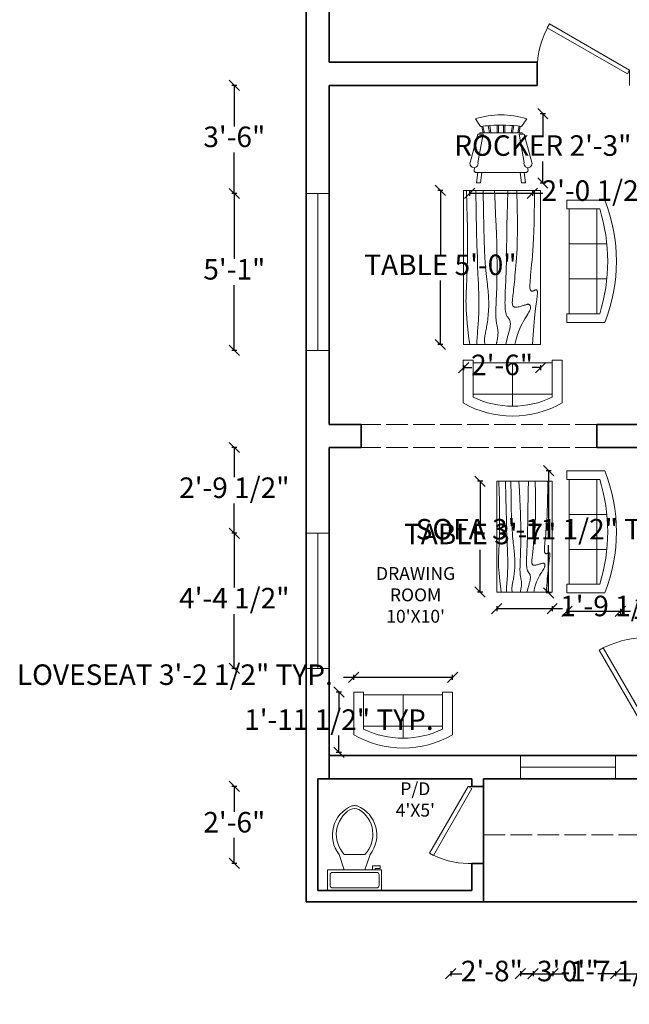
# Model space of a CAD drawing. Units: inches. Extents: x 2558 to 3026, y 433 to 1053.
# Tile 1 of 8: x 2558 to 2795, y 433 to 816. Entities that reach past the tile are written whole.
import ezdxf

# ---------------------------------------------------------------- set-up
doc = ezdxf.new("R2010")
doc.units = ezdxf.units.IN
doc.linetypes.add('ACAD_ISO02W100', pattern=[15, 12, -3])
for name, color, linetype, lineweight in [('A-ANNO-DIMS', 2, 'Continuous', 18), ('A-AREA-IDEN', 7, 'Continuous', 18), ('A-DOOR', 4, 'Continuous', 18), ('A-FLOR-FIXT', 9, 'Continuous', 18), ('A-FLOR-OVHD', 7, 'ACAD_ISO02W100', 18), ('A-FURN', 8, 'Continuous', 18), ('A-GLAZ', 5, 'Continuous', 18), ('A-WALL', 7, 'Continuous', 35), ('L-PLNT-BNDY', 253, 'ACAD_ISO02W100', 18)]:
    doc.layers.add(name, color=color, linetype=linetype, lineweight=lineweight)
doc.styles.get("Standard").update_dxf_attribs({"font": 'arial.ttf'})
doc.dimstyles.new('ISO-25', dxfattribs={"dimtxt": 8, "dimasz": 4, "dimexe": 1, "dimexo": 1, "dimgap": 1, "dimtad": 0, "dimtih": 1, "dimtoh": 1, "dimlunit": 3, "dimtxsty": 'Standard', "dimblk": 'OBLIQUE', "dimcen": 2.5, "dimclrt": 1, "dimadec": 0, "dimazin": 0, "dimtfac": 1, "dimtmove": 0, "dimatfit": 3, "dimfxl": 1, "dimfxlon": 1, "dimarcsym": 0})

# ---------------------------------------------------------------- blocks, each defined once
blk = doc.blocks.new('*U9')
for p, q in [((0, 0), (0, -6)), ((-36, 0), (-36, -6))]:
    blk.add_line(p, q)
blk.add_lwpolyline([(0, 0), (-31.18, 18), (-32.05, 16.48), (-0.88, -1.52)], close=True)
blk.add_arc((0, 0), 36, 150, 180)
blk = doc.blocks.new('*U8')
for p, q in [((0, 0), (0, -6)), ((36, 0), (36, -6))]:
    blk.add_line(p, q)
blk.add_lwpolyline([(0, 0), (31.18, 18), (32.05, 16.48), (0.87, -1.52)], close=True)
blk.add_arc((0, 0), 36, 0, 30)
blk = doc.blocks.new('*U5')
for p, q in [((0, 0), (0, 6)), ((30, 0), (30, 6))]:
    blk.add_line(p, q)
blk.add_lwpolyline([(0, 0), (25.98, -15), (26.86, -13.48), (0.87, 1.52)], close=True)
blk.add_arc((0, 0), 30, 330, 0)
blk = doc.blocks.new('Sofa - Roundback 7 ft.')
for p, q in [((-12.00002, -32.4421), (-12.00003, -6.5971)), ((11.99997, -32.4421), (11.99998, -6.5971)), ((-36.000027, -34), (-36.000027, -11.4696)), ((-35.999844, -13.3819), (35.9998, -13.3819)), ((35.99998, -34), (35.99998, -11.4696)), ((-36.000027, -32.4421), (35.99998, -32.4421))]:
    blk.add_line(p, q)
for points in [[(-36.000027, -34), (-42.000027, -34), (-42.000027, -8)], [(41.99998, -8), (41.99998, -34), (35.99998, -34)]]:
    blk.add_lwpolyline(points)
for centre, radius, start, end in [((0, -114.25), 114.25, 68.43141, 111.5686), ((-0.00001, -127.1968), 121.1968, 72.72033, 107.2797)]:
    blk.add_arc(centre, radius, start, end)
blk = doc.blocks.new('Sofa - Roundback Loveseat 5 ft.')
for p, q in [((-24, -33.99998), (-24, -11.46958)), ((0, -32.44198), (0, -5.99998)), ((24.00004, -33.99998), (24.00004, -11.46958)), ((-23.9998, -13.38178), (23.99986, -13.38178)), ((-24, -32.44198), (24.00004, -32.44198))]:
    blk.add_line(p, q)
for points in [[(-24, -33.99998), (-30, -33.99998), (-30, -7.99998)], [(30.00004, -7.99998), (30.00004, -33.99998), (24.00004, -33.99998)]]:
    blk.add_lwpolyline(points)
for centre, radius, start, end in [((0, -60.24998), 60.24998, 60.13715, 119.8628), ((0, -61.38438), 55.38444, 64.32083, 115.6792)]:
    blk.add_arc(centre, radius, start, end)
blk = doc.blocks.new('Chair - Rocking')
for p, q in [((-8, -4.5), (-10, -1.5)), ((8, -4.5), (10, -1.5)), ((-9, -7.5), (-12, -18.49999)), ((-7, -7.5), (-9, -7.5)), ((-9, -18.49999), (-7, -7.5)), ((-8.23428, -6.99939), (-8.3093, -7.47958)), ((-8.23041, -7), (8.23915, -7)), ((-7.5, -4.5), (-7, -7)), ((-6.5, -7), (-7.02225, -4.43)), ((-4.5, -7), (-4.96674, -4.19951)), ((-4, -7), (-4.40532, -4.16272)), ((-1.5, -4.05012), (-1.5, -7)), ((-1, -7), (-1, -4.05012)), ((1, -7), (1, -4.04655)), ((1.5, -4.05012), (1.5, -7)), ((4, -7), (4.40187, -4.18694)), ((4.5, -7), (4.96761, -4.19437)), ((6.5, -7), (7, -4.4057)), ((7.5, -4.5), (7, -7)), ((7, -7.5), (9, -7.5)), ((9, -18.49999), (7, -7.5)), ((8.31071, -7.48854), (8.23449, -7.00073)), ((9, -7.5), (12, -18.49999)), ((-10.36644, -20.64523), (-10.5, -21.49999)), ((-9, -22.49999), (-9.5, -26.49999)), ((0, -22.49999), (-9.5, -22.49999)), ((-8, -26.49999), (-7.5, -22.49999)), ((0, -22.49999), (9.5, -22.49999)), ((8, -26.49999), (7.5, -22.49999)), ((9, -22.49999), (9.5, -26.49999)), ((10.5, -21.49999), (10.3575, -20.58798)), ((-9.5, -26.49999), (-8, -26.49999)), ((9.5, -26.49999), (8, -26.49999))]:
    blk.add_line(p, q)
for centre, radius, start, end in [((0, -34.08333), 34.08333, 72.93847, 107.0615), ((0, -68.25004), 64.25, 93.92211, 97.15267), ((0, -68.25004), 64.25, 82.84733, 93.92211), ((-10.5, -18.99999), 1.58114, 161.5651, 18.43495), ((10.5, -18.99999), 1.58114, 161.5651, 18.43495), ((-9.5, -21.49999), 1, 180, 270), ((9.5, -21.49999), 1, 270, 0)]:
    blk.add_arc(centre, radius, start, end)
blk = doc.blocks.new('Table - Rectangular Woodgrain 60 x 30 in.')
for p, q in [((0, 0), (0, -30)), ((60, 0), (0, 0)), ((60, -30), (60, 0)), ((0, -30), (60, -30))]:
    blk.add_line(p, q)
for points in [[(0, -2.4), (4.8155, -2.418), (9.0302, -2.4688), (12.709, -2.5477), (15.9167, -2.65), (18.7181, -2.7711), (21.1781, -2.9063), (23.3616, -3.0508), (25.3333, -3.2), (27.1477, -3.3495), (28.8172, -3.4958), (30.3437, -3.636), (31.7291, -3.7667), (32.9756, -3.8849), (34.0849, -3.9875), (35.059, -4.0714), (35.9, -4.1334), (36.6114, -4.1711), (37.2041, -4.1854), (37.6906, -4.1779), (38.0833, -4.15), (38.3948, -4.1034), (38.6375, -4.0396), (38.8239, -3.9602), (38.9666, -3.8667), (39.0764, -3.7608), (39.1573, -3.6448), (39.2116, -3.521), (39.2416, -3.3917), (39.2498, -3.2593), (39.2385, -3.1261), (39.21, -2.9944), (39.1666, -2.8667), (39.111, -2.7447), (39.0468, -2.6281), (38.978, -2.5163), (38.9083, -2.4083), (38.8418, -2.3035), (38.7823, -2.201), (38.7337, -2.1001), (38.7, -2), (38.6844, -1.9003), (38.6875, -1.8021), (38.7094, -1.707), (38.75, -1.6167), (38.8094, -1.5326), (38.8875, -1.4563), (38.9844, -1.3893), (39.1, -1.3333), (39.2351, -1.2896), (39.3937, -1.2583), (39.5804, -1.2396), (39.8, -1.2333), (40.057, -1.2396), (40.3562, -1.2583), (40.7023, -1.2896), (41.1, -1.3333), (41.5547, -1.3895), (42.0755, -1.4573), (42.6721, -1.5361), (43.3542, -1.625), (44.1316, -1.7233), (45.014, -1.8302), (46.0114, -1.9449), (47.1333, -2.0667), (48.3862, -2.1947), (49.7625, -2.3281), (51.2513, -2.4663), (52.8416, -2.6083), (54.5226, -2.7535), (56.2833, -2.9011), (58.1127, -3.0501), (60, -3.2)], [(0, -9.2), (6.5759, -9.0858), (11.9385, -9.0365), (16.2527, -9.0418), (19.6833, -9.0917), (22.3952, -9.1759), (24.5531, -9.2844), (26.322, -9.4069), (27.8666, -9.5333), (29.3241, -9.6553), (30.7203, -9.7719), (32.0532, -9.8837), (33.3208, -9.9917), (34.5213, -10.0965), (35.6526, -10.199), (36.7128, -10.2999), (37.7, -10.4), (38.6129, -10.4996), (39.4531, -10.5969), (40.223, -10.6895), (40.925, -10.775), (41.5613, -10.8512), (42.1344, -10.9156), (42.6465, -10.966), (43.1, -11), (43.4976, -11.0158), (43.8437, -11.0136), (44.143, -10.9942), (44.4, -10.9583), (44.6195, -10.9069), (44.8062, -10.8406), (44.9648, -10.7603), (45.1, -10.6667), (45.2155, -10.5598), (45.3114, -10.4365), (45.3871, -10.2929), (45.4416, -10.125), (45.4743, -9.929), (45.4844, -9.7011), (45.4709, -9.4371), (45.4333, -9.1333), (45.3716, -8.7883), (45.2896, -8.4104), (45.1919, -8.0107), (45.0833, -7.6), (44.9685, -7.1893), (44.8521, -6.7896), (44.7388, -6.4117), (44.6333, -6.0667), (44.54, -5.7628), (44.4614, -5.4979), (44.4001, -5.2675), (44.3583, -5.0667), (44.3384, -4.8909), (44.3427, -4.7354), (44.3736, -4.5956), (44.4333, -4.4667), (44.5236, -4.3453), (44.6427, -4.2333), (44.7884, -4.1339), (44.9583, -4.05), (45.1501, -3.9849), (45.3614, -3.9417), (45.59, -3.9234), (45.8333, -3.9333), (46.0915, -3.9749), (46.3734, -4.0531), (46.6906, -4.1736), (47.0542, -4.3417), (47.4756, -4.5629), (47.9661, -4.8427), (48.5372, -5.1866), (49.2, -5.6), (49.9676, -6.0844), (50.8594, -6.625), (51.8965, -7.2031), (53.1, -7.8), (54.491, -8.3969), (56.0906, -8.975), (57.9199, -9.5156), (60, -10)], [(0, -12.8), (5.1847, -12.9322), (9.6213, -13.0323), (13.3963, -13.1059), (16.5958, -13.1583), (19.3063, -13.1952), (21.614, -13.2219), (23.6054, -13.2439), (25.3666, -13.2667), (26.9728, -13.2947), (28.4531, -13.3281), (29.8256, -13.3663), (31.1083, -13.4083), (32.3191, -13.4535), (33.476, -13.501), (34.597, -13.5501), (35.7, -13.6), (36.7984, -13.6497), (37.8875, -13.6979), (38.9578, -13.743), (40, -13.7833), (41.0047, -13.8174), (41.9625, -13.8438), (42.864, -13.8607), (43.7, -13.8667), (44.4631, -13.8604), (45.1552, -13.8417), (45.7801, -13.8104), (46.3416, -13.7667), (46.8439, -13.7104), (47.2906, -13.6417), (47.6858, -13.5604), (48.0333, -13.4667), (48.3375, -13.3608), (48.6042, -13.2448), (48.8396, -13.121), (49.05, -12.9917), (49.2417, -12.8593), (49.4208, -12.7261), (49.5937, -12.5944), (49.7667, -12.4667), (49.9452, -12.3451), (50.1323, -12.2313), (50.3303, -12.1268), (50.5416, -12.0333), (50.7686, -11.9524), (51.0135, -11.8854), (51.2788, -11.8341), (51.5666, -11.8), (51.8785, -11.7843), (52.2116, -11.7865), (52.562, -11.8059), (52.926, -11.8417), (53.2998, -11.8931), (53.6795, -11.9594), (54.0614, -12.0397), (54.4416, -12.1333), (54.8223, -12.2401), (55.2293, -12.3625), (55.6942, -12.5037), (56.2489, -12.6667), (56.9251, -12.8547), (57.7545, -13.0708), (58.7689, -13.3182), (60, -13.6)], [(0, -18), (5.124, -17.7273), (9.6609, -17.5057), (13.6705, -17.3303), (17.2125, -17.1958), (20.3467, -17.0973), (23.1328, -17.0297), (25.6307, -16.9878), (27.9, -16.9667), (29.9928, -16.9617), (31.9302, -16.9703), (33.7254, -16.9907), (35.3917, -17.0208), (36.9423, -17.0588), (38.3906, -17.1026), (39.7499, -17.1503), (41.0333, -17.2), (42.2519, -17.2496), (43.4073, -17.2969), (44.4986, -17.3395), (45.525, -17.375), (46.4858, -17.4012), (47.3802, -17.4156), (48.2074, -17.416), (48.9667, -17.4), (49.6583, -17.3662), (50.2872, -17.3167), (50.8595, -17.2547), (51.3812, -17.1833), (51.8584, -17.1057), (52.2971, -17.025), (52.7034, -16.9443), (53.0833, -16.8667), (53.443, -16.7951), (53.789, -16.7313), (54.128, -16.6768), (54.4666, -16.6334), (54.8115, -16.6024), (55.1693, -16.5854), (55.5465, -16.5841), (55.95, -16.6), (56.3828, -16.6337), (56.8346, -16.6823), (57.2915, -16.7418), (57.7396, -16.8084), (58.165, -16.878), (58.5539, -16.9469), (58.8924, -17.0111), (59.1666, -17.0667), (59.3679, -17.1107), (59.5078, -17.1438), (59.6032, -17.1675), (59.6708, -17.1833), (59.7275, -17.193), (59.7901, -17.1979), (59.8753, -17.1998), (60, -17.2)], [(0, -22.4), (8.0098, -22.2501), (14.4094, -22.1011), (19.4168, -21.9535), (23.25, -21.8083), (26.1269, -21.6663), (28.2656, -21.5281), (29.884, -21.3947), (31.2, -21.2667), (32.3967, -21.1448), (33.5172, -21.0292), (34.5697, -20.9198), (35.5625, -20.8167), (36.5037, -20.7198), (37.4015, -20.6292), (38.2642, -20.5448), (39.1, -20.4667), (39.9164, -20.3951), (40.7187, -20.3313), (41.5117, -20.2768), (42.3, -20.2333), (43.0883, -20.2024), (43.8812, -20.1854), (44.6836, -20.1841), (45.5, -20.2), (46.3328, -20.234), (47.1747, -20.2844), (48.0163, -20.3488), (48.8479, -20.425), (49.66, -20.5106), (50.4429, -20.6031), (51.1872, -20.7004), (51.8833, -20.8), (52.5246, -20.8999), (53.1166, -20.9995), (53.6681, -21.0983), (54.1875, -21.1958), (54.6834, -21.2919), (55.1646, -21.3859), (55.6394, -21.4777), (56.1167, -21.5667), (56.6028, -21.6515), (57.0961, -21.7266), (57.5929, -21.7852), (58.0896, -21.8208), (58.5823, -21.8268), (59.0674, -21.7964), (59.5412, -21.723), (60, -21.6)], [(0, -25.2), (8.6355, -25.0504), (15.7026, -24.9031), (21.4049, -24.7606), (25.9458, -24.625), (29.529, -24.4988), (32.3578, -24.3844), (34.6359, -24.284), (36.5667, -24.2), (38.3213, -24.1341), (39.9417, -24.0854), (41.437, -24.0523), (42.8167, -24.0333), (44.0901, -24.0268), (45.2667, -24.0313), (46.3557, -24.0451), (47.3667, -24.0667), (48.309, -24.0947), (49.1928, -24.1287), (50.0284, -24.168), (50.826, -24.2125), (51.5959, -24.2617), (52.3483, -24.3151), (53.0935, -24.3725), (53.8417, -24.4334), (54.6009, -24.497), (55.3699, -24.561), (56.1454, -24.6226), (56.9239, -24.6792), (57.7021, -24.7279), (58.4764, -24.7662), (59.2435, -24.7911), (60, -24.8)], [(0, -28.8), (5.6867, -28.6681), (10.45, -28.5698), (14.407, -28.5012), (17.675, -28.4584), (20.3711, -28.4374), (22.6125, -28.4344), (24.5164, -28.4455), (26.2, -28.4667), (27.762, -28.4947), (29.2276, -28.5281), (30.6033, -28.5663), (31.8958, -28.6084), (33.1118, -28.6535), (34.2578, -28.7011), (35.3405, -28.7501), (36.3666, -28.8), (37.3443, -28.8497), (38.288, -28.8974), (39.2137, -28.9412), (40.1375, -28.9792), (41.0753, -29.0093), (42.0432, -29.0297), (43.0572, -29.0384), (44.1333, -29.0333), (45.2936, -29.0114), (46.5843, -28.9641), (48.0579, -28.8816), (49.7666, -28.7542), (51.7629, -28.5721), (54.0989, -28.3255), (56.8272, -28.0048), (60, -27.6)]]:
    blk.add_lwpolyline(points)
blk = doc.blocks.new('Toilet - top')
for p, q in [((9.5, -6), (9.5, -2)), ((-10, -8.5), (-8, -8.5)), ((-10, -9.5), (-10, -8.5)), ((-7, -9.5), (-10, -9.5)), ((-8, -8.5), (-8, -8)), ((-7, -8), (-7, -9.5)), ((-4, -8), (-6, -14)), ((4, -8), (6, -14)), ((4, -14), (-4, -14))]:
    blk.add_line(p, q)
blk.add_lwpolyline([(10.5, -8), (10.5, 0), (-10.5, 0), (-10.5, -8)], close=True)
for points in [[(-9.5, -2), (-9.5, -6)], [(8.5, -1), (-8.5, -1)], [(-8.5, -7), (8.5, -7)]]:
    blk.add_lwpolyline(points)
for centre, radius, start, end in [((-8.62, -1.88), 0.884, 81.8699, 188.1301), ((8.62, -1.88), 0.884, 351.8699, 98.1301), ((-8.62, -6.12), 0.884, 171.8699, 278.1301), ((8.62, -6.12), 0.884, 261.8699, 8.1301), ((3.52, -21.58), 12.17, 141.4691, 247.9714), ((4.2, -21.82), 11.33, 136.3677, 238.9468), ((-3.52, -21.58), 12.17, 292.0284, 38.5307), ((-4.2, -21.82), 11.33, 301.053, 43.6321), ((0, -27.88), 4, 245.7318, 294.2682), ((0, -29), 4, 254.8605, 285.1395)]:
    blk.add_arc(centre, radius, start, end)
blk = doc.blocks.new('_Oblique')
at = {"color": 0, "linetype": 'ByBlock', "lineweight": -2}
blk.add_line((-0.5, -0.5), (0.5, 0.5), dxfattribs=at)
blk = doc.blocks.new('*D27')
at = {"layer": 'A-ANNO-DIMS', "color": 0, "lineweight": -2, "transparency": 16777216}
for p, q in [((2764.96, 640.74), (2762.96, 640.74)), ((2763.96, 640.74), (2763.96, 622.08)), ((2763.96, 593.15), (2763.96, 611.8)), ((2764.96, 593.15), (2762.96, 593.15))]:
    blk.add_line(p, q, dxfattribs=at)
at = {"layer": 'Defpoints', "color": 0, "transparency": 16777216}
for p in [(2771.1, 640.74), (2763.96, 593.15), (2771.1, 593.15)]:
    blk.add_point(p, dxfattribs=at)
at = {"layer": 'A-ANNO-DIMS', "color": 0, "lineweight": -2, "transparency": 16777216, "xscale": 4, "yscale": 4, "zscale": 4}
for p, rotation in [((2763.96, 640.74), 90), ((2763.96, 593.15), 270)]:
    blk.add_blockref('_Oblique', p, dxfattribs=dict(at, rotation=rotation))
at = {"layer": 'A-ANNO-DIMS', "color": 1, "transparency": 16777216, "insert": (2763.96, 616.94), "char_height": 8, "attachment_point": 5}
blk.add_mtext('SOFA 3\'-11 1/2" TYP.', dxfattribs=at)
blk = doc.blocks.new('*D28')
at = {"layer": 'A-ANNO-DIMS', "color": 0, "lineweight": -2, "transparency": 16777216}
for p, q in [((2771.1, 587.01), (2771.1, 585.01)), ((2791.87, 587.01), (2791.87, 585.01)), ((2771.1, 586.01), (2791.87, 586.01)), ((2791.87, 586.01), (2795.87, 586.01))]:
    blk.add_line(p, q, dxfattribs=at)
at = {"layer": 'Defpoints', "color": 0, "transparency": 16777216}
for p in [(2771.1, 593.15), (2791.87, 593.15), (2791.87, 586.01)]:
    blk.add_point(p, dxfattribs=at)
at = {"layer": 'A-ANNO-DIMS', "color": 0, "lineweight": -2, "transparency": 16777216, "xscale": 4, "yscale": 4, "zscale": 4, "rotation": 180}
blk.add_blockref('_Oblique', (2771.1, 586.01), dxfattribs=at)
at = {"layer": 'A-ANNO-DIMS', "color": 0, "lineweight": -2, "transparency": 16777216, "xscale": 4, "yscale": 4, "zscale": 4}
blk.add_blockref('_Oblique', (2791.87, 586.01), dxfattribs=at)
at = {"layer": 'A-ANNO-DIMS', "color": 1, "transparency": 16777216, "insert": (2820.88, 586.01), "char_height": 8, "attachment_point": 5}
blk.add_mtext('1\'-9" TYP.', dxfattribs=at)
blk = doc.blocks.new('*D29')
at = {"layer": 'A-ANNO-DIMS', "color": 0, "lineweight": -2, "transparency": 16777216}
for p, q in [((2688.13, 560.29), (2684.13, 560.29)), ((2688.13, 559.29), (2688.13, 561.29)), ((2726.58, 560.29), (2688.13, 560.29)), ((2726.58, 559.29), (2726.58, 561.29))]:
    blk.add_line(p, q, dxfattribs=at)
at = {"layer": 'Defpoints', "color": 0, "transparency": 16777216}
for p in [(2688.13, 560.29), (2688.13, 554.53), (2726.58, 554.53)]:
    blk.add_point(p, dxfattribs=at)
at = {"layer": 'A-ANNO-DIMS', "color": 0, "lineweight": -2, "transparency": 16777216, "xscale": 4, "yscale": 4, "zscale": 4, "rotation": 180}
blk.add_blockref('_Oblique', (2688.13, 560.29), dxfattribs=at)
at = {"layer": 'A-ANNO-DIMS', "color": 0, "lineweight": -2, "transparency": 16777216, "xscale": 4, "yscale": 4, "zscale": 4}
blk.add_blockref('_Oblique', (2726.58, 560.29), dxfattribs=at)
at = {"layer": 'A-ANNO-DIMS', "color": 1, "transparency": 16777216, "insert": (2618.55, 560.29), "char_height": 8, "attachment_point": 5}
blk.add_mtext('LOVESEAT 3\'-2 1/2" TYP.', dxfattribs=at)
blk = doc.blocks.new('*D30')
at = {"layer": 'A-ANNO-DIMS', "color": 0, "lineweight": -2, "transparency": 16777216}
for p, q in [((2683.37, 554.53), (2681.37, 554.53)), ((2682.37, 554.53), (2682.37, 547.92)), ((2682.37, 531.04), (2682.37, 537.65)), ((2683.37, 531.04), (2681.37, 531.04))]:
    blk.add_line(p, q, dxfattribs=at)
at = {"layer": 'Defpoints', "color": 0, "transparency": 16777216}
for p in [(2688.13, 554.53), (2682.37, 531.04), (2688.13, 531.04)]:
    blk.add_point(p, dxfattribs=at)
at = {"layer": 'A-ANNO-DIMS', "color": 0, "lineweight": -2, "transparency": 16777216, "xscale": 4, "yscale": 4, "zscale": 4}
for p, rotation in [((2682.37, 554.53), 90), ((2682.37, 531.04), 270)]:
    blk.add_blockref('_Oblique', p, dxfattribs=dict(at, rotation=rotation))
at = {"layer": 'A-ANNO-DIMS', "color": 1, "transparency": 16777216, "insert": (2682.37, 542.78), "char_height": 8, "attachment_point": 5}
blk.add_mtext('1\'-11 1/2" TYP.', dxfattribs=at)
blk = doc.blocks.new('*D31')
at = {"layer": 'A-ANNO-DIMS', "color": 0, "lineweight": -2, "transparency": 16777216}
for p, q in [((2722.86, 749.93), (2720.86, 749.93)), ((2721.86, 749.93), (2721.86, 725.02)), ((2721.86, 689.93), (2721.86, 714.85)), ((2722.86, 689.93), (2720.86, 689.93))]:
    blk.add_line(p, q, dxfattribs=at)
at = {"layer": 'Defpoints', "color": 0, "transparency": 16777216}
for p in [(2730.86, 749.93), (2721.86, 689.93), (2730.86, 689.93)]:
    blk.add_point(p, dxfattribs=at)
at = {"layer": 'A-ANNO-DIMS', "color": 0, "lineweight": -2, "transparency": 16777216, "xscale": 4, "yscale": 4, "zscale": 4}
for p, rotation in [((2721.86, 749.93), 90), ((2721.86, 689.93), 270)]:
    blk.add_blockref('_Oblique', p, dxfattribs=dict(at, rotation=rotation))
at = {"layer": 'A-ANNO-DIMS', "color": 1, "transparency": 16777216, "insert": (2721.86, 719.93), "char_height": 8, "attachment_point": 5}
blk.add_mtext('TABLE 5\'-0"', dxfattribs=at)
blk = doc.blocks.new('*D32')
at = {"layer": 'A-ANNO-DIMS', "color": 0, "lineweight": -2, "transparency": 16777216}
for p, q in [((2730.86, 681.93), (2730.86, 679.93)), ((2730.86, 680.93), (2734.15, 680.93)), ((2760.86, 680.93), (2757.56, 680.93)), ((2760.86, 681.93), (2760.86, 679.93))]:
    blk.add_line(p, q, dxfattribs=at)
at = {"layer": 'Defpoints', "color": 0, "transparency": 16777216}
for p in [(2730.86, 689.93), (2760.86, 689.93), (2760.86, 680.93)]:
    blk.add_point(p, dxfattribs=at)
at = {"layer": 'A-ANNO-DIMS', "color": 0, "lineweight": -2, "transparency": 16777216, "xscale": 4, "yscale": 4, "zscale": 4, "rotation": 180}
blk.add_blockref('_Oblique', (2730.86, 680.93), dxfattribs=at)
at = {"layer": 'A-ANNO-DIMS', "color": 0, "lineweight": -2, "transparency": 16777216, "xscale": 4, "yscale": 4, "zscale": 4}
blk.add_blockref('_Oblique', (2760.86, 680.93), dxfattribs=at)
at = {"layer": 'A-ANNO-DIMS', "color": 1, "transparency": 16777216, "insert": (2745.86, 680.93), "char_height": 8, "attachment_point": 5}
blk.add_mtext('2\'-6"', dxfattribs=at)
blk = doc.blocks.new('*D33')
at = {"layer": 'A-ANNO-DIMS', "color": 0, "lineweight": -2, "transparency": 16777216}
for p, q in [((2738.31, 636.64), (2736.31, 636.64)), ((2737.31, 636.64), (2737.31, 620.17)), ((2737.31, 593.52), (2737.31, 609.99)), ((2738.31, 593.52), (2736.31, 593.52))]:
    blk.add_line(p, q, dxfattribs=at)
at = {"layer": 'Defpoints', "color": 0, "transparency": 16777216}
for p in [(2743.78, 636.64), (2737.31, 593.52), (2743.78, 593.52)]:
    blk.add_point(p, dxfattribs=at)
at = {"layer": 'A-ANNO-DIMS', "color": 0, "lineweight": -2, "transparency": 16777216, "xscale": 4, "yscale": 4, "zscale": 4}
for p, rotation in [((2737.31, 636.64), 90), ((2737.31, 593.52), 270)]:
    blk.add_blockref('_Oblique', p, dxfattribs=dict(at, rotation=rotation))
at = {"layer": 'A-ANNO-DIMS', "color": 1, "transparency": 16777216, "insert": (2737.31, 615.08), "char_height": 8, "attachment_point": 5}
blk.add_mtext('TABLE 3\'-7"', dxfattribs=at)
blk = doc.blocks.new('*D34')
at = {"layer": 'A-ANNO-DIMS', "color": 0, "lineweight": -2, "transparency": 16777216}
for p, q in [((2743.78, 588.05), (2743.78, 586.05)), ((2743.78, 587.05), (2765.34, 587.05)), ((2765.34, 588.05), (2765.34, 586.05)), ((2765.34, 587.05), (2769.34, 587.05))]:
    blk.add_line(p, q, dxfattribs=at)
at = {"layer": 'Defpoints', "color": 0, "transparency": 16777216}
for p in [(2743.78, 593.52), (2765.34, 593.52), (2765.34, 587.05)]:
    blk.add_point(p, dxfattribs=at)
at = {"layer": 'A-ANNO-DIMS', "color": 0, "lineweight": -2, "transparency": 16777216, "xscale": 4, "yscale": 4, "zscale": 4, "rotation": 180}
blk.add_blockref('_Oblique', (2743.78, 587.05), dxfattribs=at)
at = {"layer": 'A-ANNO-DIMS', "color": 0, "lineweight": -2, "transparency": 16777216, "xscale": 4, "yscale": 4, "zscale": 4}
blk.add_blockref('_Oblique', (2765.34, 587.05), dxfattribs=at)
at = {"layer": 'A-ANNO-DIMS', "color": 1, "transparency": 16777216, "insert": (2789.92, 587.05), "char_height": 8, "attachment_point": 5}
blk.add_mtext('1\'-9 1/2"', dxfattribs=at)
blk = doc.blocks.new('*D39')
at = {"layer": 'A-ANNO-DIMS', "color": 0, "lineweight": -2, "transparency": 16777216}
for p, q in [((2760.72, 779.87), (2762.72, 779.87)), ((2761.72, 779.87), (2761.72, 771.51)), ((2761.72, 752.87), (2761.72, 761.23)), ((2760.72, 752.87), (2762.72, 752.87))]:
    blk.add_line(p, q, dxfattribs=at)
at = {"layer": 'Defpoints', "color": 0, "transparency": 16777216}
for p in [(2757.67, 779.87), (2761.72, 779.87), (2757.67, 752.87)]:
    blk.add_point(p, dxfattribs=at)
at = {"layer": 'A-ANNO-DIMS', "color": 0, "lineweight": -2, "transparency": 16777216, "xscale": 4, "yscale": 4, "zscale": 4}
for p, rotation in [((2761.72, 779.87), 90), ((2761.72, 752.87), 270)]:
    blk.add_blockref('_Oblique', p, dxfattribs=dict(at, rotation=rotation))
at = {"layer": 'A-ANNO-DIMS', "color": 1, "transparency": 16777216, "insert": (2761.72, 766.37), "char_height": 8, "attachment_point": 5}
blk.add_mtext('ROCKER 2\'-3"', dxfattribs=at)
blk = doc.blocks.new('*D40')
at = {"layer": 'A-ANNO-DIMS', "color": 0, "lineweight": -2, "transparency": 16777216}
for p, q in [((2733.24, 749.82), (2733.24, 747.82)), ((2733.24, 748.82), (2757.67, 748.82)), ((2757.67, 749.82), (2757.67, 747.82)), ((2757.67, 748.82), (2761.67, 748.82))]:
    blk.add_line(p, q, dxfattribs=at)
at = {"layer": 'Defpoints', "color": 0, "transparency": 16777216}
for p in [(2733.24, 752.87), (2757.67, 752.87), (2757.67, 748.82)]:
    blk.add_point(p, dxfattribs=at)
at = {"layer": 'A-ANNO-DIMS', "color": 0, "lineweight": -2, "transparency": 16777216, "xscale": 4, "yscale": 4, "zscale": 4, "rotation": 180}
blk.add_blockref('_Oblique', (2733.24, 748.82), dxfattribs=at)
at = {"layer": 'A-ANNO-DIMS', "color": 0, "lineweight": -2, "transparency": 16777216, "xscale": 4, "yscale": 4, "zscale": 4}
blk.add_blockref('_Oblique', (2757.67, 748.82), dxfattribs=at)
at = {"layer": 'A-ANNO-DIMS', "color": 1, "transparency": 16777216, "insert": (2782.69, 748.82), "char_height": 8, "attachment_point": 5}
blk.add_mtext('2\'-0 1/2"', dxfattribs=at)
blk = doc.blocks.new('*D48')
at = {"layer": 'A-ANNO-DIMS', "color": 0, "lineweight": -2, "transparency": 16777216}
for p, q in [((2725.89, 445.87), (2725.89, 443.87)), ((2725.89, 444.87), (2730.19, 444.87)), ((2757.89, 444.87), (2753.59, 444.87)), ((2757.89, 445.87), (2757.89, 443.87))]:
    blk.add_line(p, q, dxfattribs=at)
at = {"layer": 'Defpoints', "color": 0, "transparency": 16777216}
for p in [(2725.89, 943.82), (2757.89, 943.82), (2757.89, 444.87)]:
    blk.add_point(p, dxfattribs=at)
at = {"layer": 'A-ANNO-DIMS', "color": 0, "lineweight": -2, "transparency": 16777216, "xscale": 4, "yscale": 4, "zscale": 4, "rotation": 180}
blk.add_blockref('_Oblique', (2725.89, 444.87), dxfattribs=at)
at = {"layer": 'A-ANNO-DIMS', "color": 0, "lineweight": -2, "transparency": 16777216, "xscale": 4, "yscale": 4, "zscale": 4}
blk.add_blockref('_Oblique', (2757.89, 444.87), dxfattribs=at)
at = {"layer": 'A-ANNO-DIMS', "color": 1, "transparency": 16777216, "insert": (2741.89, 444.87), "char_height": 8, "attachment_point": 5}
blk.add_mtext('2\'-8"', dxfattribs=at)
blk = doc.blocks.new('*D51')
at = {"layer": 'A-ANNO-DIMS', "color": 0, "lineweight": -2, "transparency": 16777216}
for p, q in [((2642.68, 517.82), (2640.68, 517.82)), ((2641.68, 517.82), (2641.68, 507.91)), ((2641.68, 487.82), (2641.68, 497.74)), ((2642.68, 487.82), (2640.68, 487.82))]:
    blk.add_line(p, q, dxfattribs=at)
at = {"layer": 'Defpoints', "color": 0, "transparency": 16777216}
for p in [(2641.68, 517.82), (2734.13, 517.82), (2734.13, 487.82)]:
    blk.add_point(p, dxfattribs=at)
at = {"layer": 'A-ANNO-DIMS', "color": 0, "lineweight": -2, "transparency": 16777216, "xscale": 4, "yscale": 4, "zscale": 4}
for p, rotation in [((2641.68, 517.82), 90), ((2641.68, 487.82), 270)]:
    blk.add_blockref('_Oblique', p, dxfattribs=dict(at, rotation=rotation))
at = {"layer": 'A-ANNO-DIMS', "color": 1, "transparency": 16777216, "insert": (2641.68, 502.82), "char_height": 8, "attachment_point": 5}
blk.add_mtext('2\'-6"', dxfattribs=at)
blk = doc.blocks.new('*D54')
at = {"layer": 'A-ANNO-DIMS', "color": 0, "lineweight": -2, "transparency": 16777216}
for p, q in [((2642.68, 748.74), (2640.68, 748.74)), ((2641.68, 748.74), (2641.68, 723.26)), ((2641.68, 687.61), (2641.68, 713.09)), ((2642.68, 687.61), (2640.68, 687.61))]:
    blk.add_line(p, q, dxfattribs=at)
at = {"layer": 'Defpoints', "color": 0, "transparency": 16777216}
for p in [(2641.68, 748.74), (2669.63, 748.74), (2669.63, 687.61)]:
    blk.add_point(p, dxfattribs=at)
at = {"layer": 'A-ANNO-DIMS', "color": 0, "lineweight": -2, "transparency": 16777216, "xscale": 4, "yscale": 4, "zscale": 4}
for p, rotation in [((2641.68, 748.74), 90), ((2641.68, 687.61), 270)]:
    blk.add_blockref('_Oblique', p, dxfattribs=dict(at, rotation=rotation))
at = {"layer": 'A-ANNO-DIMS', "color": 1, "transparency": 16777216, "insert": (2641.68, 718.17), "char_height": 8, "attachment_point": 5}
blk.add_mtext('5\'-1"', dxfattribs=at)
blk = doc.blocks.new('*D56')
at = {"layer": 'A-ANNO-DIMS', "color": 0, "lineweight": -2, "transparency": 16777216}
for p, q in [((2642.68, 616.4), (2640.68, 616.4)), ((2641.68, 616.4), (2641.68, 595.23)), ((2641.68, 563.78), (2641.68, 584.95)), ((2642.68, 563.78), (2640.68, 563.78))]:
    blk.add_line(p, q, dxfattribs=at)
at = {"layer": 'Defpoints', "color": 0, "transparency": 16777216}
for p in [(2641.68, 616.4), (2669.63, 616.4), (2669.63, 563.78)]:
    blk.add_point(p, dxfattribs=at)
at = {"layer": 'A-ANNO-DIMS', "color": 0, "lineweight": -2, "transparency": 16777216, "xscale": 4, "yscale": 4, "zscale": 4}
for p, rotation in [((2641.68, 616.4), 90), ((2641.68, 563.78), 270)]:
    blk.add_blockref('_Oblique', p, dxfattribs=dict(at, rotation=rotation))
at = {"layer": 'A-ANNO-DIMS', "color": 1, "transparency": 16777216, "insert": (2641.68, 590.09), "char_height": 8, "attachment_point": 5}
blk.add_mtext('4\'-4 1/2"', dxfattribs=at)
blk = doc.blocks.new('*D57')
at = {"layer": 'A-ANNO-DIMS', "color": 0, "lineweight": -2, "transparency": 16777216}
for p, q in [((2752.98, 445.87), (2752.98, 443.87)), ((2752.98, 444.87), (2759.88, 444.87)), ((2790.04, 444.87), (2783.14, 444.87)), ((2790.04, 445.87), (2790.04, 443.87))]:
    blk.add_line(p, q, dxfattribs=at)
at = {"layer": 'Defpoints', "color": 0, "transparency": 16777216}
for p in [(2752.98, 520.82), (2790.04, 520.82), (2790.04, 444.87)]:
    blk.add_point(p, dxfattribs=at)
at = {"layer": 'A-ANNO-DIMS', "color": 0, "lineweight": -2, "transparency": 16777216, "xscale": 4, "yscale": 4, "zscale": 4, "rotation": 180}
blk.add_blockref('_Oblique', (2752.98, 444.87), dxfattribs=at)
at = {"layer": 'A-ANNO-DIMS', "color": 0, "lineweight": -2, "transparency": 16777216, "xscale": 4, "yscale": 4, "zscale": 4}
blk.add_blockref('_Oblique', (2790.04, 444.87), dxfattribs=at)
at = {"layer": 'A-ANNO-DIMS', "color": 1, "transparency": 16777216, "insert": (2771.51, 444.87), "char_height": 8, "attachment_point": 5}
blk.add_mtext('3\'-1"', dxfattribs=at)
blk = doc.blocks.new('*D59')
at = {"layer": 'A-ANNO-DIMS', "color": 0, "lineweight": -2, "transparency": 16777216}
for p, q in [((2690.99, 1039.77), (2690.99, 1041.77)), ((2690.99, 1040.77), (2715.93, 1040.77)), ((2782.72, 1040.77), (2757.77, 1040.77)), ((2782.72, 1039.77), (2782.72, 1041.77))]:
    blk.add_line(p, q, dxfattribs=at)
at = {"layer": 'Defpoints', "color": 0, "transparency": 16777216}
for p in [(2782.72, 1040.77), (2690.99, 658.82), (2782.72, 658.82)]:
    blk.add_point(p, dxfattribs=at)
at = {"layer": 'A-ANNO-DIMS', "color": 0, "lineweight": -2, "transparency": 16777216, "xscale": 4, "yscale": 4, "zscale": 4, "rotation": 180}
blk.add_blockref('_Oblique', (2690.99, 1040.77), dxfattribs=at)
at = {"layer": 'A-ANNO-DIMS', "color": 0, "lineweight": -2, "transparency": 16777216, "xscale": 4, "yscale": 4, "zscale": 4}
blk.add_blockref('_Oblique', (2782.72, 1040.77), dxfattribs=at)
at = {"layer": 'A-ANNO-DIMS', "color": 1, "transparency": 16777216, "insert": (2736.85, 1040.77), "char_height": 8, "attachment_point": 5}
blk.add_mtext('7\'-7 1/2"', dxfattribs=at)
blk = doc.blocks.new('*D63')
at = {"layer": 'A-ANNO-DIMS', "color": 0, "lineweight": -2, "transparency": 16777216}
for p, q in [((2757.89, 445.87), (2757.89, 443.87)), ((2757.89, 444.87), (2765.63, 444.87)), ((2765.63, 445.87), (2765.63, 443.87)), ((2765.63, 444.87), (2769.63, 444.87))]:
    blk.add_line(p, q, dxfattribs=at)
at = {"layer": 'Defpoints', "color": 0, "transparency": 16777216}
for p in [(2757.89, 943.82), (2765.63, 943.82), (2765.63, 444.87)]:
    blk.add_point(p, dxfattribs=at)
at = {"layer": 'A-ANNO-DIMS', "color": 0, "lineweight": -2, "transparency": 16777216, "xscale": 4, "yscale": 4, "zscale": 4, "rotation": 180}
blk.add_blockref('_Oblique', (2757.89, 444.87), dxfattribs=at)
at = {"layer": 'A-ANNO-DIMS', "color": 0, "lineweight": -2, "transparency": 16777216, "xscale": 4, "yscale": 4, "zscale": 4}
blk.add_blockref('_Oblique', (2765.63, 444.87), dxfattribs=at)
at = {"layer": 'A-ANNO-DIMS', "color": 1, "transparency": 16777216, "insert": (2790.59, 444.87), "char_height": 8, "attachment_point": 5}
blk.add_mtext('0\'-7 1/2"', dxfattribs=at)
blk = doc.blocks.new('*D66')
at = {"layer": 'A-ANNO-DIMS', "color": 0, "lineweight": -2, "transparency": 16777216}
for p, q in [((2642.68, 790.82), (2640.68, 790.82)), ((2641.68, 790.82), (2641.68, 774.87)), ((2641.68, 748.74), (2641.68, 764.69)), ((2642.68, 748.74), (2640.68, 748.74))]:
    blk.add_line(p, q, dxfattribs=at)
at = {"layer": 'Defpoints', "color": 0, "transparency": 16777216}
for p in [(2641.68, 790.82), (2678.63, 790.82), (2669.63, 748.74)]:
    blk.add_point(p, dxfattribs=at)
at = {"layer": 'A-ANNO-DIMS', "color": 0, "lineweight": -2, "transparency": 16777216, "xscale": 4, "yscale": 4, "zscale": 4}
for p, rotation in [((2641.68, 790.82), 90), ((2641.68, 748.74), 270)]:
    blk.add_blockref('_Oblique', p, dxfattribs=dict(at, rotation=rotation))
at = {"layer": 'A-ANNO-DIMS', "color": 1, "transparency": 16777216, "insert": (2641.68, 769.78), "char_height": 8, "attachment_point": 5}
blk.add_mtext('3\'-6"', dxfattribs=at)
blk = doc.blocks.new('*D68')
at = {"layer": 'A-ANNO-DIMS', "color": 0, "lineweight": -2, "transparency": 16777216}
for p, q in [((2642.68, 649.82), (2640.68, 649.82)), ((2641.68, 649.82), (2641.68, 638.25)), ((2641.68, 616.4), (2641.68, 627.98)), ((2642.68, 616.4), (2640.68, 616.4))]:
    blk.add_line(p, q, dxfattribs=at)
at = {"layer": 'Defpoints', "color": 0, "transparency": 16777216}
for p in [(2641.68, 649.82), (2678.63, 649.82), (2669.63, 616.4)]:
    blk.add_point(p, dxfattribs=at)
at = {"layer": 'A-ANNO-DIMS', "color": 0, "lineweight": -2, "transparency": 16777216, "xscale": 4, "yscale": 4, "zscale": 4}
for p, rotation in [((2641.68, 649.82), 90), ((2641.68, 616.4), 270)]:
    blk.add_blockref('_Oblique', p, dxfattribs=dict(at, rotation=rotation))
at = {"layer": 'A-ANNO-DIMS', "color": 1, "transparency": 16777216, "insert": (2641.68, 633.11), "char_height": 8, "attachment_point": 5}
blk.add_mtext('2\'-9 1/2"', dxfattribs=at)
blk = doc.blocks.new('*D69')
at = {"layer": 'A-ANNO-DIMS', "color": 0, "lineweight": -2, "transparency": 16777216}
for p, q in [((2790.04, 445.87), (2790.04, 443.87)), ((2790.04, 444.87), (2807.63, 444.87)), ((2807.63, 445.87), (2807.63, 443.87)), ((2807.63, 444.87), (2811.63, 444.87))]:
    blk.add_line(p, q, dxfattribs=at)
at = {"layer": 'Defpoints', "color": 0, "transparency": 16777216}
for p in [(2790.04, 520.82), (2807.63, 520.82), (2807.63, 444.87)]:
    blk.add_point(p, dxfattribs=at)
at = {"layer": 'A-ANNO-DIMS', "color": 0, "lineweight": -2, "transparency": 16777216, "xscale": 4, "yscale": 4, "zscale": 4, "rotation": 180}
blk.add_blockref('_Oblique', (2790.04, 444.87), dxfattribs=at)
at = {"layer": 'A-ANNO-DIMS', "color": 0, "lineweight": -2, "transparency": 16777216, "xscale": 4, "yscale": 4, "zscale": 4}
blk.add_blockref('_Oblique', (2807.63, 444.87), dxfattribs=at)
at = {"layer": 'A-ANNO-DIMS', "color": 1, "transparency": 16777216, "insert": (2832.21, 444.87), "char_height": 8, "attachment_point": 5}
blk.add_mtext('1\'-5 1/2"', dxfattribs=at)
blk = doc.blocks.new('*D70')
at = {"layer": 'A-ANNO-DIMS', "color": 0, "lineweight": -2, "transparency": 16777216}
for p, q in [((2678.63, 1039.77), (2678.63, 1041.77)), ((2678.63, 1040.77), (2690.99, 1040.77)), ((2690.99, 1039.77), (2690.99, 1041.77)), ((2690.99, 1040.77), (2694.99, 1040.77))]:
    blk.add_line(p, q, dxfattribs=at)
at = {"layer": 'Defpoints', "color": 0, "transparency": 16777216}
for p in [(2690.99, 1040.77), (2678.63, 658.82), (2690.99, 658.82)]:
    blk.add_point(p, dxfattribs=at)
at = {"layer": 'A-ANNO-DIMS', "color": 0, "lineweight": -2, "transparency": 16777216, "xscale": 4, "yscale": 4, "zscale": 4, "rotation": 180}
blk.add_blockref('_Oblique', (2678.63, 1040.77), dxfattribs=at)
at = {"layer": 'A-ANNO-DIMS', "color": 0, "lineweight": -2, "transparency": 16777216, "xscale": 4, "yscale": 4, "zscale": 4}
blk.add_blockref('_Oblique', (2690.99, 1040.77), dxfattribs=at)
at = {"layer": 'A-ANNO-DIMS', "color": 1, "transparency": 16777216, "insert": (2715.56, 1040.77), "char_height": 8, "attachment_point": 5}
blk.add_mtext('1\'-0 1/2"', dxfattribs=at)

msp = doc.modelspace()

# ---------------------------------------------------------------- linework, layer by layer
at = {"layer": 'A-FLOR-OVHD', "ltscale": 0.7}
for p, q in [((2782.721, 658.825), (2690.987, 658.825)), ((2782.721, 649.825), (2690.987, 649.825))]:
    msp.add_line(p, q, dxfattribs=at)
at = {"layer": 'A-GLAZ'}
for p, q in [((2678.633, 748.738), (2669.633, 748.738)), ((2674.133, 748.738), (2674.133, 687.608)), ((2678.633, 687.608), (2669.633, 687.608)), ((2678.633, 616.403), (2669.633, 616.403)), ((2674.133, 616.403), (2674.133, 563.778)), ((2678.633, 563.778), (2669.633, 563.778)), ((2752.982, 520.825), (2752.982, 529.825)), ((2790.035, 529.825), (2790.035, 520.825)), ((2752.982, 525.325), (2790.035, 525.325))]:
    msp.add_line(p, q, dxfattribs=at)
at = {"layer": 'A-WALL'}
for p, q in [((2669.633, 1012.825), (2669.633, 472.825)), ((2678.633, 943.825), (2678.633, 799.825)), ((2759.497, 799.825), (2678.633, 799.825)), ((2759.497, 790.825), (2759.497, 799.825)), ((2678.633, 790.825), (2678.633, 658.825)), ((2759.497, 790.825), (2678.633, 790.825)), ((2690.987, 658.825), (2678.633, 658.825)), ((2690.987, 658.825), (2690.987, 649.825)), ((2807.633, 658.825), (2782.721, 658.825)), ((2782.721, 649.825), (2782.721, 658.825)), ((2678.633, 649.825), (2678.633, 520.825)), ((2690.987, 649.825), (2678.633, 649.825)), ((2798.633, 649.825), (2782.721, 649.825)), ((2798.633, 529.825), (2678.633, 529.825)), ((2674.133, 520.825), (2674.133, 477.325)), ((2734.133, 520.825), (2674.133, 520.825)), ((2734.133, 520.825), (2734.133, 517.825)), ((2734.133, 517.825), (2738.633, 517.825)), ((2807.633, 520.825), (2738.633, 520.825)), ((2738.633, 520.825), (2738.633, 472.825)), ((2734.133, 487.825), (2738.633, 487.825)), ((2734.133, 487.825), (2734.133, 477.325)), ((2674.133, 477.325), (2734.133, 477.325)), ((2669.633, 472.825), (2969.633, 472.825))]:
    msp.add_line(p, q, dxfattribs=at)
at = {"layer": 'L-PLNT-BNDY', "ltscale": 0.7}
msp.add_line((2738.633, 498.947), (2960.633, 498.947), dxfattribs=at)

# ---------------------------------------------------------------- block references
at = {"layer": 'A-DOOR'}
msp.add_blockref('*U9', (2795.497, 796.825), dxfattribs=at)
for name, p, rotation in [('*U8', (2801.633, 539.691), 90), ('*U5', (2732.633, 517.825), 270)]:
    msp.add_blockref(name, p, dxfattribs=dict(at, rotation=rotation))
at = {"layer": 'A-FLOR-FIXT', "rotation": 180}
msp.add_blockref('Toilet - top', (2688.477, 477.325), dxfattribs=at)
at = {"layer": 'A-FURN'}
msp.add_blockref('Chair - Rocking', (2745.453, 779.371), dxfattribs=at)
at = {"layer": 'A-FURN', "rotation": 270}
msp.add_blockref('Table - Rectangular Woodgrain 60 x 30 in.', (2760.856, 749.933), dxfattribs=at)
at = {"layer": 'A-FURN'}
for name, p, xscale, yscale, zscale, rotation in [('Sofa - Roundback 7 ft.', (2790.362, 722.322), 0.5665475993370205, 0.5665475993370205, 0.5665475993370205, 270), ('Sofa - Roundback Loveseat 5 ft.', (2749.959, 662.045), 0.6406989062008118, 0.6406989062008118, 0.6406989062008118, 180), ('Sofa - Roundback 7 ft.', (2790.362, 616.943), 0.5665475993370205, 0.5665475993370205, 0.5665475993370205, 270), ('Table - Rectangular Woodgrain 60 x 30 in.', (2765.339, 636.641), 0.7186959398027013, 0.7186959398027013, 0.7186959398027013, 270), ('Sofa - Roundback Loveseat 5 ft.', (2707.355, 532.745), 0.6406989062008118, 0.6406989062008118, 0.6406989062008118, 180)]:
    msp.add_blockref(name, p, dxfattribs=dict(at, xscale=xscale, yscale=yscale, zscale=zscale, rotation=rotation))

# ---------------------------------------------------------------- texts
at = {"layer": 'A-AREA-IDEN', "char_height": 5, "attachment_point": 1}
for s, width, insert in [("\\pxqc;DRAWING ROOM\\P10'X10'", 50.35476, (2687.035, 603.24)), ("\\pxqc;P/D\\P4'X5'", 46.06135, (2689.073, 519.401))]:
    msp.add_mtext_dynamic_manual_height_columns(s, width=width, gutter_width=12.5, heights=[0], dxfattribs=dict(at, insert=insert))

# ---------------------------------------------------------------- dimensions: what is measured, and where the dimension line sits
at = {"layer": 'A-ANNO-DIMS'}
for base, p1, p2, picture, middle in [((2690.987, 1040.775), (2678.633, 658.825), (2690.987, 658.825), '*D70', (2715.564, 1040.775)), ((2782.721, 1040.775), (2690.987, 658.825), (2782.721, 658.825), '*D59', (2736.854, 1040.775)), ((2757.892, 444.875), (2725.892, 943.825), (2757.892, 943.825), '*D48', (2741.892, 444.875)), ((2765.633, 444.875), (2757.892, 943.825), (2765.633, 943.825), '*D63', (2790.586, 444.875)), ((2757.67, 748.821), (2733.235, 752.871), (2757.67, 752.871), '*D40', (2782.692, 748.821)), ((2760.856, 680.933), (2730.856, 689.933), (2760.856, 689.933), '*D32', (2745.856, 680.933)), ((2765.339, 587.051), (2743.778, 593.52), (2765.339, 593.52), '*D34', (2789.916, 587.051)), ((2790.035, 444.875), (2752.982, 520.825), (2790.035, 520.825), '*D57', (2771.509, 444.875)), ((2807.633, 444.875), (2790.035, 520.825), (2807.633, 520.825), '*D69', (2832.21, 444.875))]:
    dim = msp.add_linear_dim(base=base, p1=p1, p2=p2, dimstyle='ISO-25', override={"dimdec": 1, "dimlfac": 1, "dimrnd": 0, "dimzin": 1, "dimdsep": 46, "dimlunit": 4, "dimfrac": 2}, dxfattribs=at)
    dim.commit()
    dim.dimension.update_dxf_attribs({"geometry": picture, "text_midpoint": middle})
for base, p1, p2, picture, middle in [((2641.683, 790.825), (2669.633, 748.738), (2678.633, 790.825), '*D66', (2641.683, 769.781)), ((2641.683, 748.738), (2669.633, 687.608), (2669.633, 748.738), '*D54', (2641.683, 718.173)), ((2641.683, 649.825), (2669.633, 616.403), (2678.633, 649.825), '*D68', (2641.683, 633.114)), ((2641.683, 616.403), (2669.633, 563.778), (2669.633, 616.403), '*D56', (2641.683, 590.09)), ((2641.683, 517.825), (2734.133, 487.825), (2734.133, 517.825), '*D51', (2641.683, 502.825))]:
    dim = msp.add_linear_dim(base=base, p1=p1, p2=p2, angle=90, dimstyle='ISO-25', override={"dimdec": 1, "dimlfac": 1, "dimrnd": 0, "dimzin": 1, "dimdsep": 46, "dimlunit": 4, "dimfrac": 2}, dxfattribs=at)
    dim.commit()
    dim.dimension.update_dxf_attribs({"geometry": picture, "text_midpoint": middle})
for base, p1, p2, angle, text, picture, middle in [((2761.72, 779.871), (2757.67, 752.871), (2757.67, 779.871), 90, 'ROCKER <>', '*D39', (2761.72, 766.371)), ((2721.856, 689.933), (2730.856, 749.933), (2730.856, 689.933), 270, 'TABLE <>', '*D31', (2721.856, 719.933)), ((2763.96, 593.148), (2771.099, 640.738), (2771.099, 593.148), 270, 'SOFA <> TYP.', '*D27', (2763.96, 616.943)), ((2737.31, 593.52), (2743.778, 636.641), (2743.778, 593.52), 270, 'TABLE <>', '*D33', (2737.31, 615.08)), ((2688.134, 560.295), (2726.576, 554.529), (2688.134, 554.529), 180, 'LOVESEAT <> TYP.', '*D29', (2618.552, 560.295)), ((2682.367, 531.036), (2688.134, 554.529), (2688.134, 531.036), 270, '<> TYP.', '*D30', (2682.367, 542.782))]:
    dim = msp.add_linear_dim(base=base, p1=p1, p2=p2, angle=angle, text=text, dimstyle='ISO-25', override={"dimdec": 1, "dimlfac": 1, "dimrnd": 0, "dimzin": 1, "dimdsep": 46, "dimlunit": 4, "dimfrac": 2}, dxfattribs=at)
    dim.commit()
    dim.dimension.update_dxf_attribs({"geometry": picture, "text_midpoint": middle})
dim = msp.add_linear_dim(base=(2791.872, 586.009), p1=(2771.099, 593.148), p2=(2791.872, 593.148), text='<> TYP.', dimstyle='ISO-25', override={"dimdec": 1, "dimlfac": 1, "dimrnd": 0, "dimzin": 1, "dimdsep": 46, "dimlunit": 4, "dimfrac": 2}, dxfattribs=at)
dim.commit()
dim.dimension.update_dxf_attribs({"geometry": '*D28', "text_midpoint": (2820.878, 586.009)})

doc.saveas('drawing.dxf')
